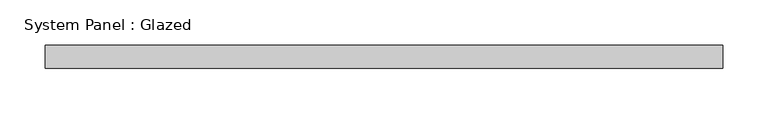
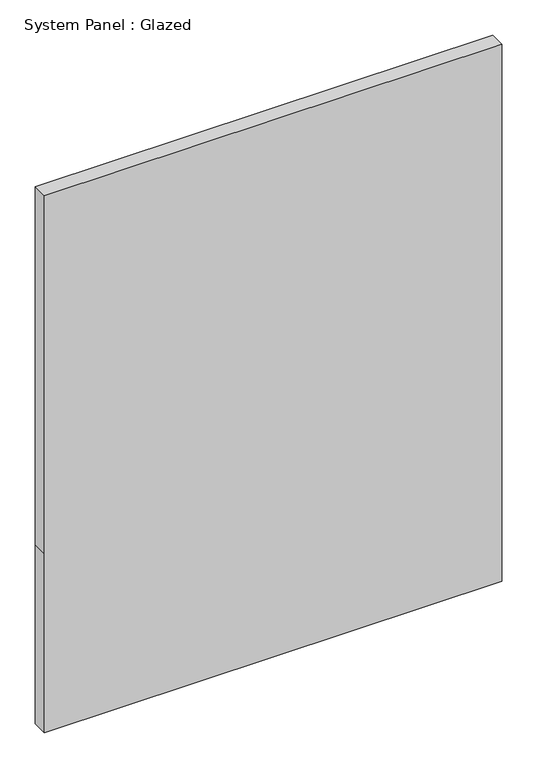
"""IFC4 building model written with IfcOpenShell, lengths in millimetres: plate geometry, System Panel : Glazed."""

from ifc_helpers import new_model, si_unit, frame, origin, place, context, project, spatial, polyline, outline, extrude, source, transform, mapped, element, save


def system_panel_glazed_aaf6793b(model_context):
    return source(origin(), model_context, "Body", "SweptSolid", [
        extrude(outline(polyline([(0.0, -374.65), (0.0, 374.65), (310.0783762, 374.65), (930.2351287, 374.65), (930.2351287, -374.65), (310.0783762, -374.65), (0.0, -374.65)])), frame((0.0, 19.05, 0.0), z_axis=(0.0, 1.0, 0.0), x_axis=(0.0, 0.0, 1.0)), (0.0, 0.0, 1.0), 25.4),
    ])


if __name__ == "__main__":
    model = new_model("IFC4")
    model_context = context("Model", 3, world=origin())
    ifc_project = project(units=[si_unit("LENGTHUNIT", "METRE", prefix="MILLI")], contexts=[model_context])
    site = spatial("IfcSite", under=ifc_project)
    building = spatial("IfcBuilding", under=site)
    placement = place(None, origin())
    system_panel_glazed_shape = system_panel_glazed_aaf6793b(model_context)
    element("IfcPlate", 1, ObjectType="System Panel : Glazed", at=placement, inside=building, context=model_context, shape_type="MappedRepresentation", body=[
        mapped(system_panel_glazed_shape, transform((0.0, 0.0, 0.0), x_axis=(1.0, 0.0, 0.0), y_axis=(0.0, 1.0, 0.0), z_axis=(0.0, 0.0, 1.0))),
    ])
    save(model, "model.ifc")

# Revit data of these elements
# Type "System Panel : Glazed"
#   Construction Type Id = "GSP4R"
#   Analytic Construction = "1/8 in Pilkington single glazing"
#   Visual Light Transmittance = 0.9
#   Solar Heat Gain Coefficient = 0.86
#   Heat Transfer Coefficient (U) = 1.18115 BTU/(h·ft²·°F)
#   Define Thermal Properties by = 1
# Element 1 (IfcPlate, "System Panel : Glazed")
#   Materials on its faces: "Glass"
# Materials
#   "Glass": class "Glass", colour RGB 0 128 192, transparency 0.75, Description = "Soda Lime Glass", Cost = 0
